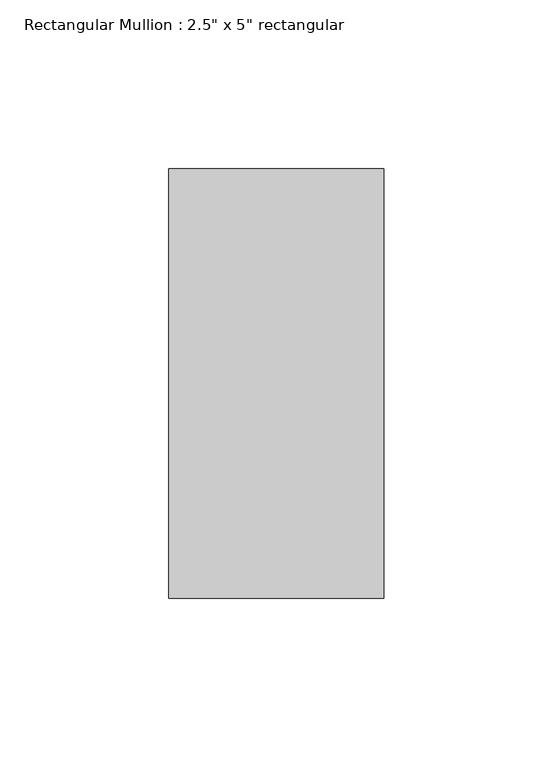
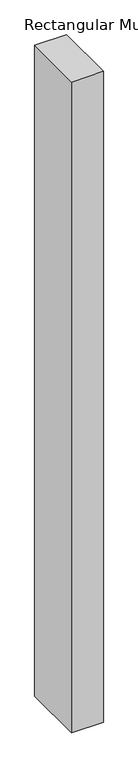
"""IFC4 building model written with IfcOpenShell, lengths in millimetres: member geometry."""

from ifc_helpers import new_model, si_unit, frame, origin, place, context, project, spatial, polyline, outline, extrude, source, transform, mapped, element, save


def member_91c435ce(model_context):
    return source(origin(), model_context, "Body", "SweptSolid", [
        extrude(outline(polyline([(0.0, 63.5), (0.0, -63.5), (-63.5, -63.5), (-63.5, 63.5), (0.0, 63.5)])), frame((0.0, 0.0, -1371.5999998), z_axis=(0.0, 0.0, 1.0), x_axis=(1.0, 0.0, 0.0)), (0.0, 0.0, 1.0), 1371.5999998),
    ])


if __name__ == "__main__":
    model = new_model("IFC4")
    model_context = context("Model", 3, world=origin())
    ifc_project = project(units=[si_unit("LENGTHUNIT", "METRE", prefix="MILLI")], contexts=[model_context])
    site = spatial("IfcSite", under=ifc_project)
    building = spatial("IfcBuilding", under=site)
    placement = place(None, origin())
    member_shape = member_91c435ce(model_context)
    element("IfcMember", 1, ObjectType="Rectangular Mullion : 2.5\" x 5\" rectangular", at=placement, inside=building, context=model_context, shape_type="MappedRepresentation", body=[
        mapped(member_shape, transform((0.0, 0.0, 0.0), x_axis=(1.0, 0.0, 0.0), y_axis=(0.0, 1.0, 0.0), z_axis=(0.0, 0.0, 1.0))),
    ])
    save(model, "model.ifc")

# Revit data of these elements
# Type "Rectangular Mullion : 2.5\" x 5\" rectangular"
#   built-in parameter 1007304 = 0.416667 (stored number, unit not read)
#   built-in parameter 1007301 = 0.104167 (stored number, unit not read)
#   built-in parameter 1007300 = 0.104167 (stored number, unit not read)
# Element 1 (IfcMember, "Rectangular Mullion : 2.5\" x 5\" rectangular")
#   Materials on its faces: "Aluminum"
# Materials
#   "Aluminum": class "Metal", colour RGB 247 247 247, transparency 0, Description = "Aluminum 6061", Cost = 0
